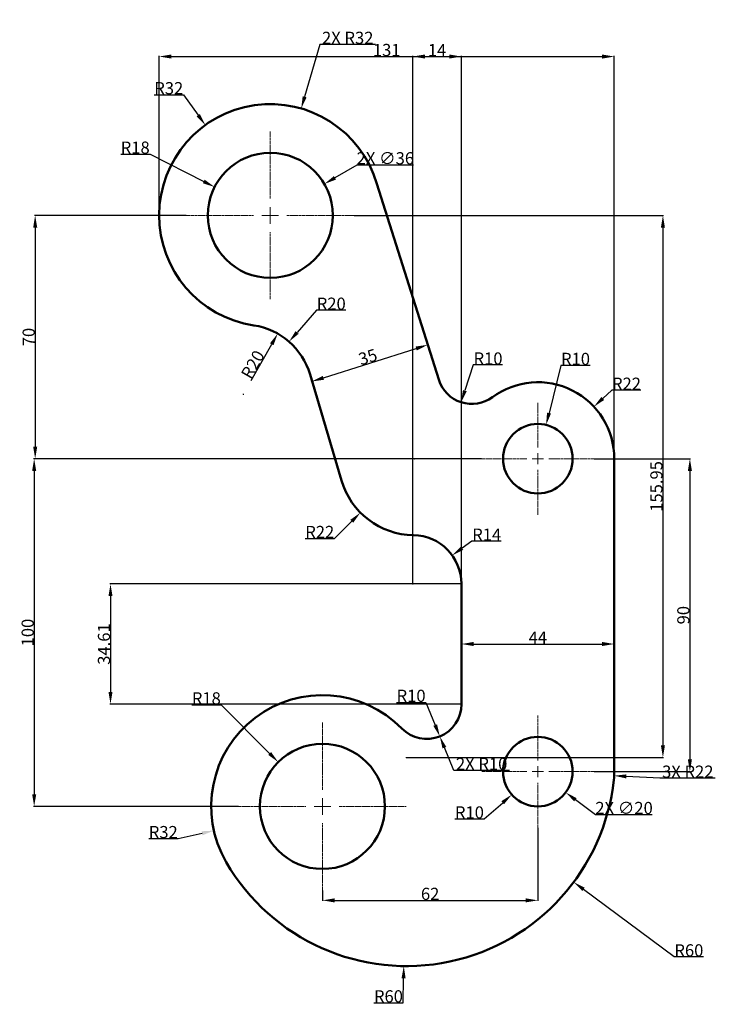
# Model space of a CAD drawing. Units: millimetres. Extents: x 104 to 305, y 97 to 381.
import ezdxf

# ---------------------------------------------------------------- set-up
doc = ezdxf.new("R2010")
doc.units = ezdxf.units.MM
doc.header["$MEASUREMENT"] = 0
doc.linetypes.add('CENTER2', pattern=[1.125, 0.75, -0.125, 0.125, -0.125])
for name, color, linetype, lineweight in [('M-CNTR', 4, 'CENTER2', 18), ('M-DIMS', 2, 'Continuous', 25), ('M-OUTL', 7, 'Continuous', 50)]:
    doc.layers.add(name, color=color, linetype=linetype, lineweight=lineweight)
doc.styles.get("Standard").update_dxf_attribs({"font": 'arial.ttf'})
doc.dimstyles.get("Standard").update_dxf_attribs({"dimtxt": 3.5, "dimasz": 3.5, "dimexe": 0.18, "dimexo": 0.0625, "dimgap": 0.09, "dimtad": 1, "dimtoh": 1, "dimdec": 0, "dimzin": 0, "dimdsep": 46, "dimtxsty": 'Standard', "dimcen": 0.09, "dimclre": 251, "dimadec": 0, "dimazin": 0, "dimtfac": 1, "dimtdec": 0, "dimtofl": 0, "dimtmove": 0, "dimatfit": 3, "dimfxl": 1, "dimtolj": 1, "dimtzin": 0, "dimarcsym": 0})

# ---------------------------------------------------------------- blocks, each defined once
blk = doc.blocks.new('*U1')
at = {"layer": 'M-CNTR', "color": 0, "transparency": 16777216}
for p, q in [((0, 4.8), (0, 24.12)), ((-24.12, 0), (-4.8, 0)), ((4.8, 0), (24.12, 0)), ((0, -24.12), (0, -4.8))]:
    blk.add_line(p, q, dxfattribs=at)
at = {"layer": 'M-CNTR', "color": 0, "linetype": 'Continuous', "transparency": 16777216}
for p, q in [((-2.4, 0), (2.4, 0)), ((0, -2.4), (0, 2.4))]:
    blk.add_line(p, q, dxfattribs=at)
blk = doc.blocks.new('*U2')
at = {"layer": 'M-CNTR', "color": 0, "transparency": 16777216}
for p, q in [((0, 3.2), (0, 16.12)), ((-16.12, 0), (-3.2, 0)), ((3.2, 0), (16.12, 0)), ((0, -16.12), (0, -3.2))]:
    blk.add_line(p, q, dxfattribs=at)
at = {"layer": 'M-CNTR', "color": 0, "linetype": 'Continuous', "transparency": 16777216}
for p, q in [((-1.6, 0), (1.6, 0)), ((0, -1.6), (0, 1.6))]:
    blk.add_line(p, q, dxfattribs=at)
blk = doc.blocks.new('*U3')
at = {"layer": 'M-CNTR', "color": 0, "transparency": 16777216}
for p, q in [((0, 3.2), (0, 16.12)), ((-16.12, 0), (-3.2, 0)), ((3.2, 0), (16.12, 0)), ((0, -16.12), (0, -3.2))]:
    blk.add_line(p, q, dxfattribs=at)
at = {"layer": 'M-CNTR', "color": 0, "linetype": 'Continuous', "transparency": 16777216}
for p, q in [((-1.6, 0), (1.6, 0)), ((0, -1.6), (0, 1.6))]:
    blk.add_line(p, q, dxfattribs=at)
blk = doc.blocks.new('*U4')
at = {"layer": 'M-CNTR', "color": 0, "transparency": 16777216}
for p, q in [((0, 4.8), (0, 24.12)), ((-24.12, 0), (-4.8, 0)), ((4.8, 0), (24.12, 0)), ((0, -24.12), (0, -4.8))]:
    blk.add_line(p, q, dxfattribs=at)
at = {"layer": 'M-CNTR', "color": 0, "linetype": 'Continuous', "transparency": 16777216}
for p, q in [((-2.4, 0), (2.4, 0)), ((0, -2.4), (0, 2.4))]:
    blk.add_line(p, q, dxfattribs=at)
blk = doc.blocks.new('*D5')
at = {"layer": 'Defpoints', "color": 0, "transparency": 16777216}
for p in [(157.93, 350.34), (176.63, 324.36)]:
    blk.add_point(p, dxfattribs=at)
at = {"layer": 'M-DIMS', "color": 0, "lineweight": -2, "transparency": 16777216}
for p, q in [((143.24, 359.06), (151.66, 359.06)), ((151.66, 359.06), (155.89, 353.18)), ((176.54, 324.36), (176.72, 324.36)), ((176.63, 324.27), (176.63, 324.45))]:
    blk.add_line(p, q, dxfattribs=at)
at = {"layer": 'M-DIMS', "color": 0, "transparency": 16777216}
blk.add_solid([(156.36, 353.52), (155.42, 352.84), (157.93, 350.34)], dxfattribs=at)
at = {"layer": 'M-DIMS', "color": 0, "transparency": 16777216, "insert": (147.4, 360.94), "char_height": 3.5, "attachment_point": 5}
blk.add_mtext('\\A1;R32', dxfattribs=at)
blk = doc.blocks.new('*D6')
at = {"layer": 'Defpoints', "color": 0, "transparency": 16777216}
for p in [(160.58, 332.52), (176.63, 324.36)]:
    blk.add_point(p, dxfattribs=at)
at = {"layer": 'M-DIMS', "color": 0, "lineweight": -2, "transparency": 16777216}
for p, q in [((133.57, 341.96), (142.03, 341.96)), ((142.03, 341.96), (157.47, 334.11)), ((176.54, 324.36), (176.72, 324.36)), ((176.63, 324.27), (176.63, 324.45))]:
    blk.add_line(p, q, dxfattribs=at)
at = {"layer": 'M-DIMS', "color": 0, "transparency": 16777216}
blk.add_solid([(157.73, 334.63), (157.2, 333.59), (160.58, 332.52)], dxfattribs=at)
at = {"layer": 'M-DIMS', "color": 0, "transparency": 16777216, "insert": (137.75, 343.84), "char_height": 3.5, "attachment_point": 5}
blk.add_mtext('\\A1;R18', dxfattribs=at)
blk = doc.blocks.new('*D7')
at = {"layer": 'Defpoints', "color": 0, "transparency": 16777216}
for p in [(178.76, 290.34), (168.89, 272.94)]:
    blk.add_point(p, dxfattribs=at)
at = {"layer": 'M-DIMS', "color": 0, "lineweight": -2, "transparency": 16777216}
blk.add_line((171.09, 276.83), (177.03, 287.29), dxfattribs=at)
at = {"layer": 'M-DIMS', "color": 0, "transparency": 16777216}
blk.add_solid([(176.53, 287.58), (177.54, 287.01), (178.76, 290.34)], dxfattribs=at)
at = {"layer": 'M-DIMS', "color": 0, "transparency": 16777216, "insert": (171.57, 281.47), "char_height": 3.5, "attachment_point": 5, "rotation": 60.4189}
blk.add_mtext('\\A1;R20', dxfattribs=at)
blk = doc.blocks.new('*D8')
at = {"layer": 'Defpoints', "color": 0, "transparency": 16777216}
for p in [(234.64, 280.12), (231.55, 270.61)]:
    blk.add_point(p, dxfattribs=at)
at = {"layer": 'M-DIMS', "color": 0, "lineweight": -2, "transparency": 16777216}
for p, q in [((235.03, 281.33), (232.63, 273.94)), ((243.48, 281.33), (235.03, 281.33))]:
    blk.add_line(p, q, dxfattribs=at)
at = {"layer": 'M-DIMS', "color": 0, "transparency": 16777216}
blk.add_solid([(232.08, 274.12), (233.18, 273.76), (231.55, 270.61)], dxfattribs=at)
at = {"layer": 'M-DIMS', "color": 0, "transparency": 16777216, "insert": (239.3, 283.2), "char_height": 3.5, "attachment_point": 5}
blk.add_mtext('\\A1;R10', dxfattribs=at)
blk = doc.blocks.new('*D9')
at = {"layer": 'Defpoints', "color": 0, "transparency": 16777216}
for p in [(269.76, 269.32), (253.63, 254.36)]:
    blk.add_point(p, dxfattribs=at)
at = {"layer": 'M-DIMS', "color": 0, "lineweight": -2, "transparency": 16777216}
for p, q in [((274.9, 274.08), (272.33, 271.7)), ((283.31, 274.08), (274.9, 274.08)), ((253.54, 254.36), (253.72, 254.36)), ((253.63, 254.27), (253.63, 254.45))]:
    blk.add_line(p, q, dxfattribs=at)
at = {"layer": 'M-DIMS', "color": 0, "transparency": 16777216}
blk.add_solid([(271.93, 272.13), (272.73, 271.27), (269.76, 269.32)], dxfattribs=at)
at = {"layer": 'M-DIMS', "color": 0, "transparency": 16777216, "insert": (279.15, 275.93), "char_height": 3.5, "attachment_point": 5}
blk.add_mtext('\\A1;R22', dxfattribs=at)
blk = doc.blocks.new('*D10')
at = {"layer": 'Defpoints', "color": 0, "transparency": 16777216}
for p in [(256.01, 264.08), (253.63, 254.36)]:
    blk.add_point(p, dxfattribs=at)
at = {"layer": 'M-DIMS', "color": 0, "lineweight": -2, "transparency": 16777216}
for p, q in [((260.21, 281.19), (256.85, 267.47)), ((268.66, 281.19), (260.21, 281.19)), ((253.54, 254.36), (253.72, 254.36)), ((253.63, 254.27), (253.63, 254.45))]:
    blk.add_line(p, q, dxfattribs=at)
at = {"layer": 'M-DIMS', "color": 0, "transparency": 16777216}
blk.add_solid([(256.28, 267.61), (257.41, 267.34), (256.01, 264.08)], dxfattribs=at)
at = {"layer": 'M-DIMS', "color": 0, "transparency": 16777216, "insert": (264.48, 283.07), "char_height": 3.5, "attachment_point": 5}
blk.add_mtext('\\A1;R10', dxfattribs=at)
blk = doc.blocks.new('*D11')
at = {"layer": 'Defpoints', "color": 0, "transparency": 16777216}
for p in [(228.97, 226.57), (217.63, 218.37)]:
    blk.add_point(p, dxfattribs=at)
at = {"layer": 'M-DIMS', "color": 0, "lineweight": -2, "transparency": 16777216}
for p, q in [((234.64, 230.68), (231.81, 228.62)), ((243.08, 230.68), (234.64, 230.68)), ((217.54, 218.37), (217.72, 218.37)), ((217.63, 218.28), (217.63, 218.46))]:
    blk.add_line(p, q, dxfattribs=at)
at = {"layer": 'M-DIMS', "color": 0, "transparency": 16777216}
blk.add_solid([(231.47, 229.1), (232.15, 228.15), (228.97, 226.57)], dxfattribs=at)
at = {"layer": 'M-DIMS', "color": 0, "transparency": 16777216, "insert": (238.91, 232.52), "char_height": 3.5, "attachment_point": 5}
blk.add_mtext('\\A1;R14', dxfattribs=at)
blk = doc.blocks.new('*D12')
at = {"layer": 'Defpoints', "color": 0, "transparency": 16777216}
for p in [(218.18, 254.36), (202.57, 238.85)]:
    blk.add_point(p, dxfattribs=at)
at = {"layer": 'M-DIMS', "color": 0, "lineweight": -2, "transparency": 16777216}
for p, q in [((218.09, 254.36), (218.27, 254.36)), ((218.18, 254.27), (218.18, 254.45)), ((195.12, 231.44), (200.09, 236.38)), ((186.7, 231.44), (195.12, 231.44))]:
    blk.add_line(p, q, dxfattribs=at)
at = {"layer": 'M-DIMS', "color": 0, "transparency": 16777216}
blk.add_solid([(199.68, 236.8), (200.5, 235.97), (202.57, 238.85)], dxfattribs=at)
at = {"layer": 'M-DIMS', "color": 0, "transparency": 16777216, "insert": (190.86, 233.29), "char_height": 3.5, "attachment_point": 5}
blk.add_mtext('\\A1;R22', dxfattribs=at)
blk = doc.blocks.new('*D13')
at = {"layer": 'Defpoints', "color": 0, "transparency": 16777216}
for p in [(178.91, 167.1), (191.63, 154.36)]:
    blk.add_point(p, dxfattribs=at)
at = {"layer": 'M-DIMS', "color": 0, "lineweight": -2, "transparency": 16777216}
for p, q in [((154.04, 183.55), (162.5, 183.55)), ((162.5, 183.55), (176.44, 169.58)), ((191.54, 154.36), (191.72, 154.36)), ((191.63, 154.27), (191.63, 154.45))]:
    blk.add_line(p, q, dxfattribs=at)
at = {"layer": 'M-DIMS', "color": 0, "transparency": 16777216}
blk.add_solid([(176.85, 169.99), (176.03, 169.17), (178.91, 167.1)], dxfattribs=at)
at = {"layer": 'M-DIMS', "color": 0, "transparency": 16777216, "insert": (158.22, 185.43), "char_height": 3.5, "attachment_point": 5}
blk.add_mtext('\\A1;R18', dxfattribs=at)
blk = doc.blocks.new('*D14')
at = {"layer": 'Defpoints', "color": 0, "transparency": 16777216}
for p in [(191.63, 154.36), (160.4, 147.39)]:
    blk.add_point(p, dxfattribs=at)
at = {"layer": 'M-DIMS', "color": 0, "lineweight": -2, "transparency": 16777216}
for p, q in [((191.54, 154.36), (191.72, 154.36)), ((191.63, 154.27), (191.63, 154.45)), ((141.66, 145.09), (150.08, 145.09)), ((150.08, 145.09), (156.98, 146.63))]:
    blk.add_line(p, q, dxfattribs=at)
at = {"layer": 'M-DIMS', "color": 0, "transparency": 16777216}
blk.add_solid([(156.85, 147.2), (157.11, 146.06), (160.4, 147.39)], dxfattribs=at)
at = {"layer": 'M-DIMS', "color": 0, "transparency": 16777216, "insert": (145.82, 146.97), "char_height": 3.5, "attachment_point": 5}
blk.add_mtext('\\A1;R32', dxfattribs=at)
blk = doc.blocks.new('*D15')
at = {"layer": 'Defpoints', "color": 0, "transparency": 16777216}
for p in [(215.85, 168.42), (215.04, 108.42)]:
    blk.add_point(p, dxfattribs=at)
at = {"layer": 'M-DIMS', "color": 0, "lineweight": -2, "transparency": 16777216}
for p, q in [((215.76, 168.42), (215.94, 168.42)), ((215.85, 168.33), (215.85, 168.51)), ((214.89, 97.85), (214.99, 104.92)), ((206.45, 97.85), (214.89, 97.85))]:
    blk.add_line(p, q, dxfattribs=at)
at = {"layer": 'M-DIMS', "color": 0, "transparency": 16777216}
blk.add_solid([(214.41, 104.93), (215.57, 104.92), (215.04, 108.42)], dxfattribs=at)
at = {"layer": 'M-DIMS', "color": 0, "transparency": 16777216, "insert": (210.63, 99.73), "char_height": 3.5, "attachment_point": 5}
blk.add_mtext('\\A1;R60', dxfattribs=at)
blk = doc.blocks.new('*D16')
at = {"layer": 'Defpoints', "color": 0, "transparency": 16777216}
for p in [(221.95, 287.12), (223.21, 283.13), (189.85, 272.59)]:
    blk.add_point(p, dxfattribs=at)
at = {"layer": 'M-DIMS', "color": 0, "lineweight": -2, "transparency": 16777216}
for p, q in [((191.92, 277.64), (218.61, 286.07)), ((223.19, 283.19), (221.89, 287.29)), ((189.83, 272.65), (188.53, 276.76))]:
    blk.add_line(p, q, dxfattribs=at)
at = {"layer": 'M-DIMS', "color": 0, "transparency": 16777216}
for points in [[(218.43, 286.62), (218.78, 285.51), (221.95, 287.12)], [(191.75, 278.2), (192.1, 277.08), (188.59, 276.58)]]:
    blk.add_solid(points, dxfattribs=at)
at = {"layer": 'M-DIMS', "color": 0, "transparency": 16777216, "insert": (204.7, 283.64), "char_height": 3.5, "attachment_point": 5, "rotation": 17.5291}
blk.add_mtext('\\A1;35', dxfattribs=at)
blk = doc.blocks.new('*D17')
at = {"layer": 'Defpoints', "color": 0, "transparency": 16777216}
for p in [(152.51, 324.36), (108.95, 254.36), (237.51, 254.36)]:
    blk.add_point(p, dxfattribs=at)
at = {"layer": 'M-DIMS', "color": 0, "lineweight": -2, "transparency": 16777216}
for p, q in [((152.45, 324.36), (108.77, 324.36)), ((108.95, 320.86), (108.95, 257.86)), ((237.45, 254.36), (108.77, 254.36))]:
    blk.add_line(p, q, dxfattribs=at)
at = {"layer": 'M-DIMS', "color": 0, "transparency": 16777216}
for points in [[(108.37, 320.86), (109.54, 320.86), (108.95, 324.36)], [(108.37, 257.86), (109.54, 257.86), (108.95, 254.36)]]:
    blk.add_solid(points, dxfattribs=at)
at = {"layer": 'M-DIMS', "color": 0, "transparency": 16777216, "insert": (107.08, 289.36), "char_height": 3.5, "attachment_point": 5, "rotation": 90}
blk.add_mtext('\\A1;70', dxfattribs=at)
blk = doc.blocks.new('*D18')
at = {"layer": 'Defpoints', "color": 0, "transparency": 16777216}
for p in [(237.51, 254.36), (108.66, 154.36), (167.51, 154.36)]:
    blk.add_point(p, dxfattribs=at)
at = {"layer": 'M-DIMS', "color": 0, "lineweight": -2, "transparency": 16777216}
for p, q in [((237.45, 254.36), (108.48, 254.36)), ((108.66, 250.86), (108.66, 157.86)), ((167.45, 154.36), (108.48, 154.36))]:
    blk.add_line(p, q, dxfattribs=at)
at = {"layer": 'M-DIMS', "color": 0, "transparency": 16777216}
for points in [[(108.08, 250.86), (109.25, 250.86), (108.66, 254.36)], [(108.08, 157.86), (109.25, 157.86), (108.66, 154.36)]]:
    blk.add_solid(points, dxfattribs=at)
at = {"layer": 'M-DIMS', "color": 0, "transparency": 16777216, "insert": (106.79, 204.36), "char_height": 3.5, "attachment_point": 5, "rotation": 90}
blk.add_mtext('\\A1;100', dxfattribs=at)
blk = doc.blocks.new('*D19')
at = {"layer": 'Defpoints', "color": 0, "transparency": 16777216}
for p in [(269.75, 254.36), (269.75, 164.36), (297.39, 164.36)]:
    blk.add_point(p, dxfattribs=at)
at = {"layer": 'M-DIMS', "color": 0, "lineweight": -2, "transparency": 16777216}
for p, q in [((269.81, 254.36), (297.57, 254.36)), ((297.39, 250.86), (297.39, 167.86)), ((269.81, 164.36), (297.57, 164.36))]:
    blk.add_line(p, q, dxfattribs=at)
at = {"layer": 'M-DIMS', "color": 0, "transparency": 16777216}
for points in [[(296.81, 250.86), (297.98, 250.86), (297.39, 254.36)], [(296.81, 167.86), (297.98, 167.86), (297.39, 164.36)]]:
    blk.add_solid(points, dxfattribs=at)
at = {"layer": 'M-DIMS', "color": 0, "transparency": 16777216, "insert": (295.51, 209.36), "char_height": 3.5, "attachment_point": 5, "rotation": 90}
blk.add_mtext('\\A1;90', dxfattribs=at)
blk = doc.blocks.new('*D20')
at = {"layer": 'Defpoints', "color": 0, "transparency": 16777216}
for p in [(231.63, 201.06), (275.63, 201.06), (275.63, 201.06)]:
    blk.add_point(p, dxfattribs=at)
at = {"layer": 'M-DIMS', "color": 0, "lineweight": -2, "transparency": 16777216}
for p, q in [((231.63, 201.13), (231.63, 201.24)), ((275.63, 201.13), (275.63, 201.24)), ((235.13, 201.06), (272.13, 201.06))]:
    blk.add_line(p, q, dxfattribs=at)
at = {"layer": 'M-DIMS', "color": 0, "transparency": 16777216}
for points in [[(235.13, 201.65), (235.13, 200.48), (231.63, 201.06)], [(272.13, 201.65), (272.13, 200.48), (275.63, 201.06)]]:
    blk.add_solid(points, dxfattribs=at)
at = {"layer": 'M-DIMS', "color": 0, "transparency": 16777216, "insert": (253.63, 202.9), "char_height": 3.5, "attachment_point": 5}
blk.add_mtext('\\A1;44', dxfattribs=at)
blk = doc.blocks.new('*D21')
at = {"layer": 'Defpoints', "color": 0, "transparency": 16777216}
for p in [(221.63, 183.76), (225.41, 174.5)]:
    blk.add_point(p, dxfattribs=at)
at = {"layer": 'M-DIMS', "color": 0, "lineweight": -2, "transparency": 16777216}
for p, q in [((212.97, 184.29), (221.41, 184.29)), ((221.41, 184.29), (224.09, 177.74))]:
    blk.add_line(p, q, dxfattribs=at)
at = {"layer": 'M-DIMS', "color": 0, "transparency": 16777216}
blk.add_solid([(224.63, 177.96), (223.55, 177.52), (225.41, 174.5)], dxfattribs=at)
at = {"layer": 'M-DIMS', "color": 0, "transparency": 16777216, "insert": (217.15, 186.17), "char_height": 3.5, "attachment_point": 5}
blk.add_mtext('\\A1;R10', dxfattribs=at)
blk = doc.blocks.new('*D22')
at = {"layer": 'Defpoints', "color": 0, "transparency": 16777216}
for p in [(253.63, 148.24), (191.63, 130.24), (253.63, 127.33)]:
    blk.add_point(p, dxfattribs=at)
at = {"layer": 'M-DIMS', "color": 0, "lineweight": -2, "transparency": 16777216}
for p, q in [((253.63, 148.18), (253.63, 127.15)), ((191.63, 130.18), (191.63, 127.15)), ((195.13, 127.33), (250.13, 127.33))]:
    blk.add_line(p, q, dxfattribs=at)
at = {"layer": 'M-DIMS', "color": 0, "transparency": 16777216}
for points in [[(195.13, 127.91), (195.13, 126.74), (191.63, 127.33)], [(250.13, 127.91), (250.13, 126.74), (253.63, 127.33)]]:
    blk.add_solid(points, dxfattribs=at)
at = {"layer": 'M-DIMS', "color": 0, "transparency": 16777216, "insert": (222.63, 129.2), "char_height": 3.5, "attachment_point": 5}
blk.add_mtext('\\A1;62', dxfattribs=at)
blk = doc.blocks.new('*D23')
at = {"layer": 'Defpoints', "color": 0, "transparency": 16777216}
for p in [(253.63, 164.36), (246.13, 157.74)]:
    blk.add_point(p, dxfattribs=at)
at = {"layer": 'M-DIMS', "color": 0, "lineweight": -2, "transparency": 16777216}
for p, q in [((253.54, 164.36), (253.72, 164.36)), ((253.63, 164.27), (253.63, 164.45)), ((238.21, 150.74), (243.51, 155.43)), ((229.77, 150.74), (238.21, 150.74))]:
    blk.add_line(p, q, dxfattribs=at)
at = {"layer": 'M-DIMS', "color": 0, "transparency": 16777216}
blk.add_solid([(243.13, 155.86), (243.9, 154.99), (246.13, 157.74)], dxfattribs=at)
at = {"layer": 'M-DIMS', "color": 0, "transparency": 16777216, "insert": (233.94, 152.62), "char_height": 3.5, "attachment_point": 5}
blk.add_mtext('\\A1;R10', dxfattribs=at)
blk = doc.blocks.new('*D24')
at = {"layer": 'Defpoints', "color": 0, "transparency": 16777216}
for p in [(275.63, 370.04), (144.63, 324.49), (275.63, 254.36)]:
    blk.add_point(p, dxfattribs=at)
at = {"layer": 'M-DIMS', "color": 251, "lineweight": -2, "transparency": 16777216}
for p, q in [((144.63, 324.55), (144.63, 370.22)), ((275.63, 254.43), (275.63, 370.22))]:
    blk.add_line(p, q, dxfattribs=at)
at = {"layer": 'M-DIMS', "color": 0, "lineweight": -2, "transparency": 16777216}
blk.add_line((148.13, 370.04), (272.13, 370.04), dxfattribs=at)
at = {"layer": 'M-DIMS', "color": 0, "transparency": 16777216}
for points in [[(148.13, 370.63), (148.13, 369.46), (144.63, 370.04)], [(272.13, 370.63), (272.13, 369.46), (275.63, 370.04)]]:
    blk.add_solid(points, dxfattribs=at)
at = {"layer": 'M-DIMS', "color": 0, "transparency": 16777216, "insert": (210.13, 371.92), "char_height": 3.5, "attachment_point": 5}
blk.add_mtext('\\A1;131', dxfattribs=at)
blk = doc.blocks.new('*D25')
at = {"layer": 'Defpoints', "color": 0, "transparency": 16777216}
for p in [(200.75, 324.36), (215.85, 168.42), (289.63, 168.42)]:
    blk.add_point(p, dxfattribs=at)
at = {"layer": 'M-DIMS', "color": 251, "lineweight": -2, "transparency": 16777216}
for p, q in [((200.81, 324.36), (289.81, 324.36)), ((215.91, 168.42), (289.81, 168.42))]:
    blk.add_line(p, q, dxfattribs=at)
at = {"layer": 'M-DIMS', "color": 0, "lineweight": -2, "transparency": 16777216}
blk.add_line((289.63, 320.86), (289.63, 171.92), dxfattribs=at)
at = {"layer": 'M-DIMS', "color": 0, "transparency": 16777216}
for points in [[(289.05, 320.86), (290.21, 320.86), (289.63, 324.36)], [(289.05, 171.92), (290.21, 171.92), (289.63, 168.42)]]:
    blk.add_solid(points, dxfattribs=at)
at = {"layer": 'M-DIMS', "color": 0, "transparency": 16777216, "insert": (287.75, 246.39), "char_height": 3.5, "attachment_point": 5, "rotation": 90}
blk.add_mtext('\\A1;155.95', dxfattribs=at)
blk = doc.blocks.new('*D26')
at = {"layer": 'Defpoints', "color": 0, "transparency": 16777216}
for p in [(231.63, 218.37), (130.63, 183.76), (231.63, 183.76)]:
    blk.add_point(p, dxfattribs=at)
at = {"layer": 'M-DIMS', "color": 251, "lineweight": -2, "transparency": 16777216}
for p, q in [((231.57, 218.37), (130.45, 218.37)), ((231.57, 183.76), (130.45, 183.76))]:
    blk.add_line(p, q, dxfattribs=at)
at = {"layer": 'M-DIMS', "color": 0, "lineweight": -2, "transparency": 16777216}
blk.add_line((130.63, 214.87), (130.63, 187.26), dxfattribs=at)
at = {"layer": 'M-DIMS', "color": 0, "transparency": 16777216}
for points in [[(130.05, 214.87), (131.21, 214.87), (130.63, 218.37)], [(130.05, 187.26), (131.21, 187.26), (130.63, 183.76)]]:
    blk.add_solid(points, dxfattribs=at)
at = {"layer": 'M-DIMS', "color": 0, "transparency": 16777216, "insert": (128.75, 201.06), "char_height": 3.5, "attachment_point": 5, "rotation": 90}
blk.add_mtext('\\A1;34.61', dxfattribs=at)
blk = doc.blocks.new('*D27')
at = {"layer": 'Defpoints', "color": 0, "transparency": 16777216}
for p in [(231.63, 370.04), (217.63, 218.37), (231.63, 218.37)]:
    blk.add_point(p, dxfattribs=at)
at = {"layer": 'M-DIMS', "color": 251, "lineweight": -2, "transparency": 16777216}
for p, q in [((217.63, 218.43), (217.63, 370.22)), ((231.63, 218.43), (231.63, 370.22))]:
    blk.add_line(p, q, dxfattribs=at)
at = {"layer": 'M-DIMS', "color": 0, "lineweight": -2, "transparency": 16777216}
blk.add_line((221.13, 370.04), (228.13, 370.04), dxfattribs=at)
at = {"layer": 'M-DIMS', "color": 0, "transparency": 16777216}
for points in [[(221.13, 370.63), (221.13, 369.46), (217.63, 370.04)], [(228.13, 370.63), (228.13, 369.46), (231.63, 370.04)]]:
    blk.add_solid(points, dxfattribs=at)
at = {"layer": 'M-DIMS', "color": 0, "transparency": 16777216, "insert": (224.63, 371.89), "char_height": 3.5, "attachment_point": 5}
blk.add_mtext('\\A1;14', dxfattribs=at)
blk = doc.blocks.new('*D28')
at = {"layer": 'Defpoints', "color": 0, "transparency": 16777216}
for p in [(192.2, 333.4), (161.06, 315.33)]:
    blk.add_point(p, dxfattribs=at)
at = {"layer": 'M-DIMS', "color": 0, "lineweight": -2, "transparency": 16777216}
for p, q in [((201.54, 338.82), (195.23, 335.16)), ((217.84, 338.82), (201.54, 338.82))]:
    blk.add_line(p, q, dxfattribs=at)
at = {"layer": 'M-DIMS', "color": 251, "lineweight": -2, "transparency": 16777216}
for p, q in [((176.54, 324.36), (176.72, 324.36)), ((176.63, 324.27), (176.63, 324.45))]:
    blk.add_line(p, q, dxfattribs=at)
at = {"layer": 'M-DIMS', "color": 0, "transparency": 16777216}
blk.add_solid([(194.93, 335.66), (195.52, 334.65), (192.2, 333.4)], dxfattribs=at)
at = {"layer": 'M-DIMS', "color": 0, "transparency": 16777216, "insert": (209.74, 340.79), "char_height": 3.5, "attachment_point": 5}
blk.add_mtext('\\A1;2X ∅36', dxfattribs=at)
blk = doc.blocks.new('*D29')
at = {"layer": 'Defpoints', "color": 0, "transparency": 16777216}
for p in [(245.62, 170.36), (261.64, 158.37)]:
    blk.add_point(p, dxfattribs=at)
at = {"layer": 'M-DIMS', "color": 251, "lineweight": -2, "transparency": 16777216}
for p, q in [((253.54, 164.36), (253.72, 164.36)), ((253.63, 164.27), (253.63, 164.45))]:
    blk.add_line(p, q, dxfattribs=at)
at = {"layer": 'M-DIMS', "color": 0, "lineweight": -2, "transparency": 16777216}
for p, q in [((270.26, 151.92), (264.44, 156.28)), ((286.55, 151.92), (270.26, 151.92))]:
    blk.add_line(p, q, dxfattribs=at)
at = {"layer": 'M-DIMS', "color": 0, "transparency": 16777216}
blk.add_solid([(264.79, 156.74), (264.09, 155.81), (261.64, 158.37)], dxfattribs=at)
at = {"layer": 'M-DIMS', "color": 0, "transparency": 16777216, "insert": (278.45, 153.9), "char_height": 3.5, "attachment_point": 5}
blk.add_mtext('\\A1;2X ∅20', dxfattribs=at)
blk = doc.blocks.new('*D30')
at = {"layer": 'Defpoints', "color": 0, "transparency": 16777216}
for p in [(185.53, 355.1), (176.63, 324.36)]:
    blk.add_point(p, dxfattribs=at)
at = {"layer": 'M-DIMS', "color": 0, "lineweight": -2, "transparency": 16777216}
for p, q in [((190.87, 373.54), (186.5, 358.46)), ((206.87, 373.54), (190.87, 373.54))]:
    blk.add_line(p, q, dxfattribs=at)
at = {"layer": 'M-DIMS', "color": 251, "lineweight": -2, "transparency": 16777216}
for p, q in [((176.54, 324.36), (176.72, 324.36)), ((176.63, 324.27), (176.63, 324.45))]:
    blk.add_line(p, q, dxfattribs=at)
at = {"layer": 'M-DIMS', "color": 0, "transparency": 16777216}
blk.add_solid([(185.94, 358.63), (187.06, 358.3), (185.53, 355.1)], dxfattribs=at)
at = {"layer": 'M-DIMS', "color": 0, "transparency": 16777216, "insert": (198.91, 375.42), "char_height": 3.5, "attachment_point": 5}
blk.add_mtext('\\A1;2X R32', dxfattribs=at)
blk = doc.blocks.new('*D31')
at = {"layer": 'Defpoints', "color": 0, "transparency": 16777216}
for p in [(253.63, 164.36), (275.6, 163.18)]:
    blk.add_point(p, dxfattribs=at)
at = {"layer": 'M-DIMS', "color": 251, "lineweight": -2, "transparency": 16777216}
for p, q in [((253.54, 164.36), (253.72, 164.36)), ((253.63, 164.27), (253.63, 164.45))]:
    blk.add_line(p, q, dxfattribs=at)
at = {"layer": 'M-DIMS', "color": 0, "lineweight": -2, "transparency": 16777216}
for p, q in [((288.78, 162.47), (279.09, 162.99)), ((304.71, 162.47), (288.78, 162.47))]:
    blk.add_line(p, q, dxfattribs=at)
at = {"layer": 'M-DIMS', "color": 0, "transparency": 16777216}
blk.add_solid([(279.12, 163.57), (279.06, 162.41), (275.6, 163.18)], dxfattribs=at)
at = {"layer": 'M-DIMS', "color": 0, "transparency": 16777216, "insert": (296.79, 164.35), "char_height": 3.5, "attachment_point": 5}
blk.add_mtext('\\A1;3X R22', dxfattribs=at)
blk = doc.blocks.new('*D32')
at = {"layer": 'Defpoints', "color": 0, "transparency": 16777216}
for p in [(182.02, 288.03), (168.89, 272.94)]:
    blk.add_point(p, dxfattribs=at)
at = {"layer": 'M-DIMS', "color": 0, "lineweight": -2, "transparency": 16777216}
for p, q in [((189.9, 297.08), (184.32, 290.67)), ((198.34, 297.08), (189.9, 297.08))]:
    blk.add_line(p, q, dxfattribs=at)
at = {"layer": 'M-DIMS', "color": 251, "lineweight": -2, "transparency": 16777216}
for p, q in [((168.8, 272.94), (168.98, 272.94)), ((168.89, 272.85), (168.89, 273.03))]:
    blk.add_line(p, q, dxfattribs=at)
at = {"layer": 'M-DIMS', "color": 0, "transparency": 16777216}
blk.add_solid([(183.88, 291.05), (184.76, 290.28), (182.02, 288.03)], dxfattribs=at)
at = {"layer": 'M-DIMS', "color": 0, "transparency": 16777216, "insert": (194.17, 298.95), "char_height": 3.5, "attachment_point": 5}
blk.add_mtext('\\A1;R20', dxfattribs=at)
blk = doc.blocks.new('*D33')
at = {"layer": 'Defpoints', "color": 0, "transparency": 16777216}
for p in [(221.63, 183.76), (225.41, 174.5)]:
    blk.add_point(p, dxfattribs=at)
at = {"layer": 'M-DIMS', "color": 251, "lineweight": -2, "transparency": 16777216}
for p, q in [((221.54, 183.76), (221.72, 183.76)), ((221.63, 183.67), (221.63, 183.85))]:
    blk.add_line(p, q, dxfattribs=at)
at = {"layer": 'M-DIMS', "color": 0, "lineweight": -2, "transparency": 16777216}
for p, q in [((229.41, 164.71), (226.73, 171.26)), ((245.43, 164.71), (229.41, 164.71))]:
    blk.add_line(p, q, dxfattribs=at)
at = {"layer": 'M-DIMS', "color": 0, "transparency": 16777216}
blk.add_solid([(227.27, 171.48), (226.19, 171.04), (225.41, 174.5)], dxfattribs=at)
at = {"layer": 'M-DIMS', "color": 0, "transparency": 16777216, "insert": (237.46, 166.59), "char_height": 3.5, "attachment_point": 5}
blk.add_mtext('\\A1;2X R10', dxfattribs=at)
blk = doc.blocks.new('*D34')
at = {"layer": 'Defpoints', "color": 0, "transparency": 16777216}
for p in [(215.85, 168.42), (263.97, 132.58)]:
    blk.add_point(p, dxfattribs=at)
at = {"layer": 'M-DIMS', "color": 251, "lineweight": -2, "transparency": 16777216}
for p, q in [((215.76, 168.42), (215.94, 168.42)), ((215.85, 168.33), (215.85, 168.51))]:
    blk.add_line(p, q, dxfattribs=at)
at = {"layer": 'M-DIMS', "color": 0, "lineweight": -2, "transparency": 16777216}
for p, q in [((292.84, 111.08), (266.77, 130.49)), ((301.28, 111.08), (292.84, 111.08))]:
    blk.add_line(p, q, dxfattribs=at)
at = {"layer": 'M-DIMS', "color": 0, "transparency": 16777216}
blk.add_solid([(267.12, 130.96), (266.43, 130.02), (263.97, 132.58)], dxfattribs=at)
at = {"layer": 'M-DIMS', "color": 0, "transparency": 16777216, "insert": (297.1, 112.95), "char_height": 3.5, "attachment_point": 5}
blk.add_mtext('\\A1;R60', dxfattribs=at)

msp = doc.modelspace()

# ---------------------------------------------------------------- linework, layer by layer
at = {"layer": 'M-OUTL'}
for p, q in [((225.107, 277.111), (207.317, 333.435)), ((197.078, 248.128), (188.067, 278.613)), ((275.629, 254.364), (275.629, 164.364)), ((231.629, 218.368), (231.629, 183.758))]:
    msp.add_line(p, q, dxfattribs=at)
for centre, radius in [((176.629, 324.364), 18), ((253.629, 254.364), 10), ((253.629, 164.364), 10), ((191.629, 154.364), 18)]:
    msp.add_circle(centre, radius, dxfattribs=at)
for centre, radius, start, end in [((176.629, 324.364), 32, 16.46654, 261.43754), ((168.887, 272.944), 20, 16.46654, 81.43754), ((234.643, 280.123), 10, 197.52912, 306.39361), ((253.629, 254.364), 22, 0, 126.39361), ((218.175, 254.364), 22, 196.46654, 269.1312), ((217.629, 218.368), 14, 0, 89.1312), ((191.629, 154.364), 32, 44.41531, 210.12969), ((221.629, 183.758), 10, 224.41531, 0), ((253.629, 164.364), 22, 353.8745, 0), ((215.846, 168.419), 60, 210.12969, 353.8745)]:
    msp.add_arc(centre, radius, start, end, dxfattribs=at)

# ---------------------------------------------------------------- block references
at = {"layer": 'M-CNTR'}
for name, p in [('*U4', (176.629, 324.364)), ('*U3', (253.629, 254.364)), ('*U1', (191.629, 154.364)), ('*U2', (253.629, 164.364))]:
    msp.add_blockref(name, p, dxfattribs=at)

# ---------------------------------------------------------------- dimensions: what is measured, and where the dimension line sits
at = {"layer": 'M-DIMS'}
for center, mpoint, text, picture, middle in [((176.629, 324.364), (185.529, 355.102), '2X <>', '*D30', (198.913, 373.544)), ((253.629, 164.364), (275.597, 163.18), '3X <>', '*D31', (288.778, 162.469))]:
    dim = msp.add_radius_dim(center=center, mpoint=mpoint, text=text, dimstyle='Standard', override={"dimdec": 0, "dimlfac": 1, "dimrnd": 0, "dimzin": 0, "dimdsep": 46, "dimlunit": 2}, dxfattribs=at)
    dim.commit()
    dim.dimension.update_dxf_attribs({"geometry": picture, "text_midpoint": middle, "dimtype": 164})
for base, p1, p2, override, picture, middle in [((275.629, 370.043), (144.63, 324.487), (275.629, 254.364), {"dimdec": 0, "dimlfac": 1, "dimrnd": 0, "dimzin": 0, "dimdsep": 46, "dimlunit": 2}, '*D24', (210.129, 371.921)), ((231.629, 370.043), (217.629, 218.368), (231.629, 218.368), {"dimdec": 0, "dimlfac": 1, "dimrnd": 0, "dimzin": 0, "dimdsep": 46, "dimlunit": 2}, '*D27', (224.629, 371.89)), ((275.629, 201.063), (231.629, 201.063), (275.629, 201.063), {"dimclrd": 0, "dimclre": 0, "dimclrt": 0}, '*D20', (253.629, 202.903)), ((253.629, 127.328), (191.629, 130.244), (253.629, 148.244), {"dimclrd": 0, "dimclre": 0, "dimclrt": 0}, '*D22', (222.629, 129.205))]:
    dim = msp.add_linear_dim(base=base, p1=p1, p2=p2, dimstyle='Standard', override=override, dxfattribs=at)
    dim.commit()
    dim.dimension.update_dxf_attribs({"geometry": picture, "text_midpoint": middle})
for center, mpoint, override, picture, middle in [((176.629, 324.364), (157.935, 350.336), {"dimclrd": 0, "dimclre": 0, "dimclrt": 0}, '*D5', (147.403, 359.057)), ((176.629, 324.364), (160.585, 332.523), {"dimclrd": 0, "dimclre": 0, "dimclrt": 0}, '*D6', (137.752, 341.961)), ((168.887, 272.944), (182.021, 288.027), {"dimdec": 0, "dimlfac": 1, "dimrnd": 0, "dimzin": 0, "dimdsep": 46, "dimlunit": 2}, '*D32', (194.167, 297.077)), ((168.887, 272.944), (178.76, 290.337), {"dimclrd": 0, "dimclre": 0, "dimclrt": 0}, '*D7', (173.199, 280.54)), ((234.643, 280.123), (231.546, 270.614), {"dimclrd": 0, "dimclre": 0, "dimclrt": 0}, '*D8', (239.3, 281.326)), ((253.629, 254.364), (256.013, 264.076), {"dimclrd": 0, "dimclre": 0, "dimclrt": 0}, '*D10', (264.48, 281.188)), ((191.629, 154.364), (178.913, 167.104), {"dimclrd": 0, "dimclre": 0, "dimclrt": 0}, '*D13', (158.223, 183.55)), ((221.629, 183.758), (225.409, 174.5), {"dimclrd": 0, "dimclre": 0, "dimclrt": 0}, '*D21', (217.147, 184.29)), ((215.846, 168.419), (263.967, 132.58), {"dimdec": 0, "dimlfac": 1, "dimrnd": 0, "dimzin": 0, "dimdsep": 46, "dimlunit": 2}, '*D34', (297.104, 111.077))]:
    dim = msp.add_radius_dim(center=center, mpoint=mpoint, dimstyle='Standard', override=override, dxfattribs=at)
    dim.commit()
    dim.dimension.update_dxf_attribs({"geometry": picture, "text_midpoint": middle, "dimtype": 164})
for p1, p2, picture, middle in [((161.061, 315.33), (192.198, 333.399), '*D28', (209.736, 338.819)), ((245.623, 170.355), (261.636, 158.373), '*D29', (278.451, 151.921))]:
    dim = msp.add_diameter_dim_2p(p1=p1, p2=p2, text='2X <>', dimstyle='Standard', override={"dimdec": 0, "dimlfac": 1, "dimrnd": 0, "dimzin": 0, "dimdsep": 46, "dimlunit": 2}, dxfattribs=at)
    dim.commit()
    dim.dimension.update_dxf_attribs({"geometry": picture, "text_midpoint": middle, "dimtype": 163})
for base, p1, p2, override, picture, middle in [((108.954, 254.364), (152.509, 324.364), (237.509, 254.364), {"dimclrd": 0, "dimclre": 0, "dimclrt": 0}, '*D17', (107.077, 289.364)), ((289.6294, 168.4191), (200.7494, 324.3642), (215.8463, 168.4191), {"dimdec": 2, "dimlfac": 1, "dimrnd": 0, "dimzin": 0, "dimdsep": 46, "dimlunit": 2}, '*D25', (287.7524, 246.3917)), ((108.662, 154.364), (237.509, 254.364), (167.509, 154.364), {"dimclrd": 0, "dimclre": 0, "dimclrt": 0}, '*D18', (106.785, 204.364)), ((297.392, 164.364), (269.749, 254.364), (269.749, 164.364), {"dimclrd": 0, "dimclre": 0, "dimclrt": 0}, '*D19', (295.515, 209.364)), ((130.63, 183.758), (231.629, 218.368), (231.629, 183.758), {"dimdec": 2, "dimlfac": 1, "dimrnd": 0, "dimzin": 0, "dimdsep": 46, "dimlunit": 2}, '*D26', (128.751, 201.063))]:
    dim = msp.add_linear_dim(base=base, p1=p1, p2=p2, angle=90, dimstyle='Standard', override=override, dxfattribs=at)
    dim.commit()
    dim.dimension.update_dxf_attribs({"geometry": picture, "text_midpoint": middle})
dim = msp.add_aligned_dim(p1=(189.846, 272.593), p2=(223.206, 283.13), distance=4.186, dimstyle='Standard', override={"dimclrd": 0, "dimclre": 0, "dimclrt": 0}, dxfattribs=at)
dim.commit()
dim.dimension.update_dxf_attribs({"geometry": '*D16', "text_midpoint": (204.7, 283.644)})
for center, mpoint, picture, middle in [((253.629, 254.364), (269.764, 269.32), '*D9', (279.151, 275.926)), ((218.175, 254.364), (202.574, 238.853), '*D12', (190.865, 233.286)), ((217.629, 218.368), (228.973, 226.574), '*D11', (238.909, 232.523)), ((215.846, 168.419), (215.037, 108.425), '*D15', (210.629, 99.729)), ((253.629, 164.364), (246.135, 157.744), '*D23', (233.944, 152.621)), ((191.629, 154.364), (160.398, 147.395), '*D14', (145.821, 146.97))]:
    dim = msp.add_radius_dim(center=center, mpoint=mpoint, dimstyle='Standard', override={"dimclrd": 0, "dimclre": 0, "dimclrt": 0}, dxfattribs=at)
    dim.commit()
    dim.dimension.update_dxf_attribs({"geometry": picture, "text_midpoint": middle})
dim = msp.add_radius_dim(center=(221.629, 183.758), mpoint=(225.409, 174.5), text='2X <>', dimstyle='Standard', override={"dimdec": 0, "dimlfac": 1, "dimrnd": 0, "dimzin": 0, "dimdsep": 46, "dimlunit": 2}, dxfattribs=at)
dim.commit()
dim.dimension.update_dxf_attribs({"geometry": '*D33', "text_midpoint": (237.461, 166.587)})

doc.saveas('drawing.dxf')
